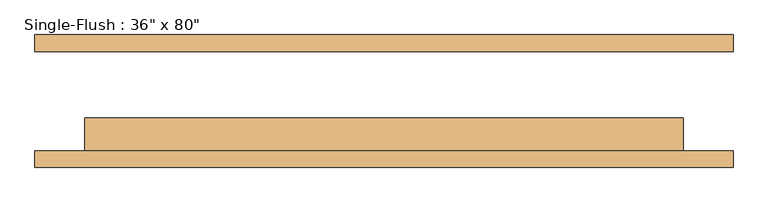
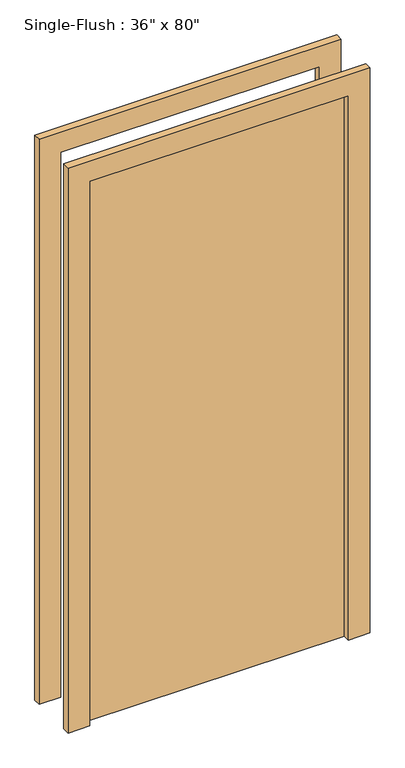
"""IFC4 building model written with IfcOpenShell, lengths in millimetres: door geometry."""

from ifc_helpers import new_model, si_unit, frame, origin, origin_with_axes, place, context, project, spatial, polyline, outline, extrude, source, transform, mapped, element, save


def door_2b0b55a0(model_context):
    return source(origin(), model_context, "Body", "SweptSolid", [
        extrude(outline(polyline([(2108.2, -533.4), (0.0, -533.4), (0.0, -457.2), (2032.0, -457.2), (2032.0, 457.2), (0.0, 457.2), (0.0, 533.4), (2108.2, 533.4), (2108.2, -533.4)])), frame((0.0, -101.6, 0.0), z_axis=(0.0, 1.0, 0.0), x_axis=(0.0, 0.0, 1.0)), (0.0, 0.0, 1.0), 25.4),
        extrude(outline(polyline([(2108.2, 533.4), (2108.2, -533.4), (0.0, -533.4), (0.0, -457.2), (2032.0, -457.2), (2032.0, 457.2), (0.0, 457.2), (0.0, 533.4), (2108.2, 533.4)])), frame((0.0, 76.2, 0.0), z_axis=(0.0, 1.0, 0.0), x_axis=(0.0, 0.0, 1.0)), (0.0, 0.0, 1.0), 25.4),
        extrude(outline(polyline([(457.2, -25.4), (457.2, -76.2), (-457.2, -76.2), (-457.2, -25.4), (457.2, -25.4)])), origin_with_axes(), (0.0, 0.0, 1.0), 2032.0),
    ])


if __name__ == "__main__":
    model = new_model("IFC4")
    model_context = context("Model", 3, world=origin())
    ifc_project = project(units=[si_unit("LENGTHUNIT", "METRE", prefix="MILLI")], contexts=[model_context])
    site = spatial("IfcSite", under=ifc_project)
    building = spatial("IfcBuilding", under=site)
    placement = place(None, origin())
    door_shape = door_2b0b55a0(model_context)
    element("IfcDoor", 1, ObjectType="Single-Flush : 36\" x 80\"", at=placement, inside=building, context=model_context, shape_type="MappedRepresentation", body=[
        mapped(door_shape, transform((0.0, 0.0, 0.0), x_axis=(1.0, 0.0, 0.0), y_axis=(0.0, 1.0, 0.0), z_axis=(0.0, 0.0, 1.0))),
    ])
    save(model, "model.ifc")

# Revit data of these elements
# Type "Single-Flush : 36\" x 80\""
#   Type Mark = "6"
#   Construction Type Id = "MDOOR"
#   Assembly Code = "C1020"
#   Analytic Construction = "Metal"
#   Thickness = 0' - 2"
#   Heat Transfer Coefficient (U) = 0.651978 BTU/(h·ft²·°F)
#   Height = 6' - 8"
#   Trim Projection Ext = 0' - 1"
#   Trim Projection Int = 0' - 1"
#   Trim Width = 0' - 3"
#   Width = 3' - 0"
#   Define Thermal Properties by = 1
#   Door Material = Door - Panel
#   Frame Material = Door - Frame
#   Visual Light Transmittance = 0
#   Solar Heat Gain Coefficient = 0
#   Function = (empty or 0)
#   Wall Closure = (empty or 0)
# Element 1 (IfcDoor, "Single-Flush : 36\" x 80\"")
#   Materials on its faces: "Door - Frame", "Door - Panel"
# Materials
#   "Door - Panel": class "Wood", colour RGB 210 159 95, transparency 0
#   "Door - Frame": colour RGB 118 70 51, transparency 0
